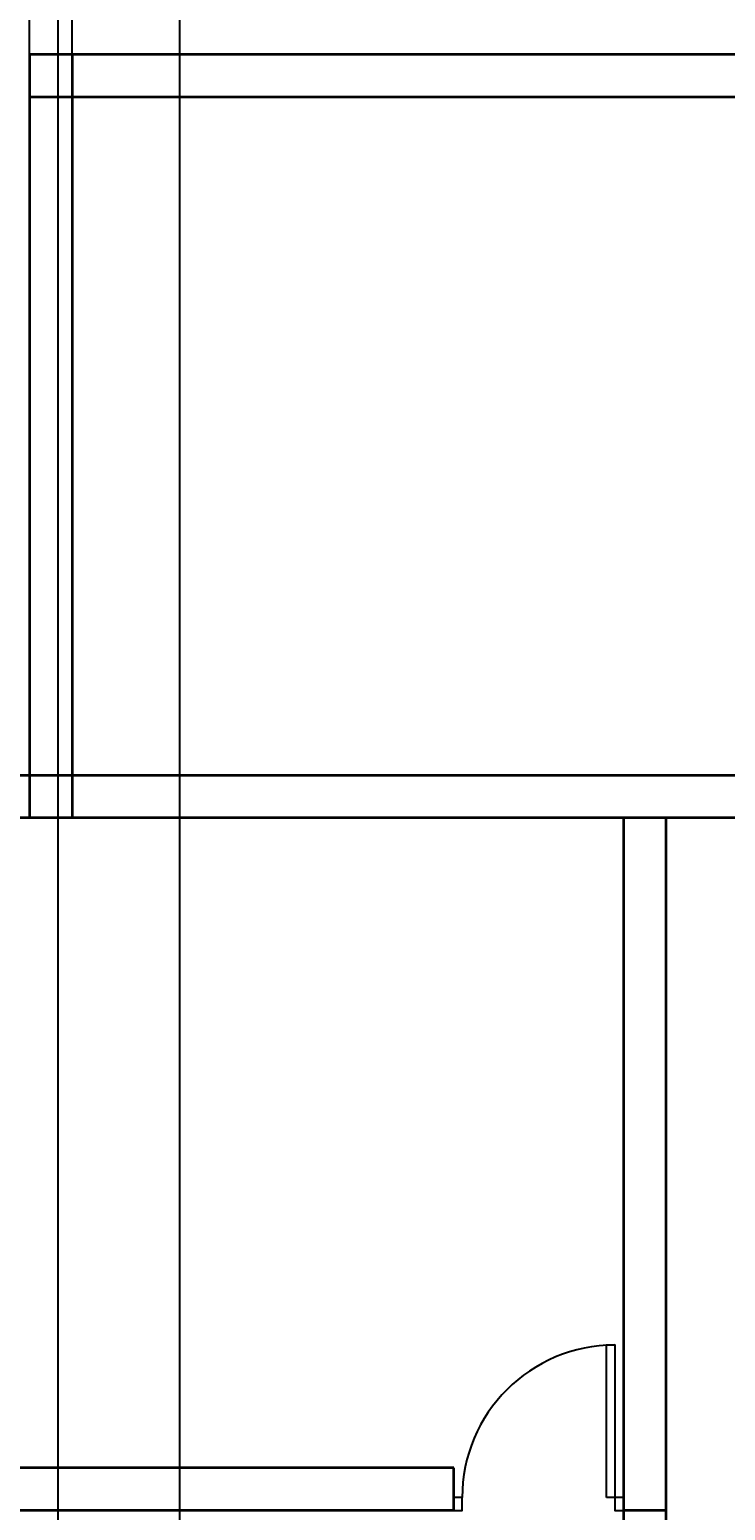
# Model space of a CAD drawing. Units: inches. Extents: x 867 to 1667, y -234 to 788.
# Tile 28 of 42: x 1071 to 1219, y 258 to 572. Entities that reach past the tile are written whole.
import ezdxf

# ---------------------------------------------------------------- set-up
doc = ezdxf.new("R2010")
doc.units = ezdxf.units.IN
doc.header["$MEASUREMENT"] = 0
for name, color, linetype, lineweight in [('A-ANNO-DIMS', 2, 'Continuous', 18), ('A-Door', 150, 'Continuous', 25), ('A-Wall', 7, 'Continuous', 35)]:
    doc.layers.add(name, color=color, linetype=linetype, lineweight=lineweight)
doc.layers.add('NET 01', color=8, linetype='Continuous')
doc.styles.get("Standard").update_dxf_attribs({"font": 'arial.ttf'})
doc.dimstyles.get("Standard").update_dxf_attribs({"dimtxt": 0.6875, "dimasz": 0.18, "dimexe": 0.18, "dimexo": 0.0625, "dimgap": 0.09, "dimtad": 0, "dimdec": 4, "dimzin": 0, "dimdsep": 46, "dimlunit": 4, "dimtxsty": 'Standard', "dimcen": 0.09, "dimadec": 0, "dimazin": 0, "dimtfac": 1, "dimtdec": 4, "dimtofl": 0, "dimtmove": 0, "dimatfit": 3, "dimfxl": 1, "dimtolj": 1, "dimtzin": 0, "dimarcsym": 0})

# ---------------------------------------------------------------- blocks, each defined once
blk = doc.blocks.new('A$C292B336C')
at = {"layer": 'A-Door'}
for points in [[(-0.05, 0), (-0.05, 0.9), (0, 0.9), (0, 0)], [(-0.95, 0), (-0.95, -0.075), (-0.9, -0.075), (-0.9, 0)], [(0, 0), (0, -0.075), (0.05, -0.075), (0.05, 0)]]:
    blk.add_lwpolyline(points, close=True, dxfattribs=at)
at = {"layer": 'NET 01'}
blk.add_arc((0, 0), 0.9, 90, 180, dxfattribs=at)
blk = doc.blocks.new('*D29')
at = {"layer": 'A-ANNO-DIMS', "color": 0, "lineweight": -2, "transparency": 16777216}
for p, q in [((1076.89, 623.55), (1076.89, -233.54)), ((1102.67, 623.55), (1102.67, -233.54)), ((1077.07, -233.36), (1088.52, -233.36)), ((1102.49, -233.36), (1091.03, -233.36))]:
    blk.add_line(p, q, dxfattribs=at)
at = {"layer": 'A-ANNO-DIMS', "color": 0, "transparency": 16777216}
for points in [[(1077.07, -233.33), (1077.07, -233.39), (1076.89, -233.36)], [(1102.49, -233.33), (1102.49, -233.39), (1102.67, -233.36)]]:
    blk.add_solid(points, dxfattribs=at)
at = {"layer": 'Defpoints', "color": 0, "transparency": 16777216}
for p in [(1076.89, 623.62), (1102.67, 623.62), (1102.67, -233.36)]:
    blk.add_point(p, dxfattribs=at)
at = {"layer": 'A-ANNO-DIMS', "color": 0, "transparency": 16777216, "insert": (1089.78, -233.36), "char_height": 0.688, "attachment_point": 5}
blk.add_mtext('\\A1;25.78', dxfattribs=at)
blk = doc.blocks.new('*D31')
at = {"layer": 'A-ANNO-DIMS', "color": 0, "lineweight": -2, "transparency": 16777216}
for p, q in [((1070.89, 566.68), (1070.89, 787.75)), ((1071.07, 787.57), (1304.02, 787.57)), ((1538.71, 787.57), (1305.75, 787.57)), ((1538.89, 566.68), (1538.89, 787.75))]:
    blk.add_line(p, q, dxfattribs=at)
at = {"layer": 'A-ANNO-DIMS', "color": 0, "transparency": 16777216}
for points in [[(1071.07, 787.6), (1071.07, 787.54), (1070.89, 787.57)], [(1538.71, 787.6), (1538.71, 787.54), (1538.89, 787.57)]]:
    blk.add_solid(points, dxfattribs=at)
at = {"layer": 'Defpoints', "color": 0, "transparency": 16777216}
for p in [(1538.89, 787.57), (1070.89, 566.62), (1538.89, 566.62)]:
    blk.add_point(p, dxfattribs=at)
at = {"layer": 'A-ANNO-DIMS', "color": 0, "transparency": 16777216, "insert": (1304.89, 787.57), "char_height": 0.688, "attachment_point": 5}
blk.add_mtext('\\A1;468', dxfattribs=at)
blk = doc.blocks.new('*D32')
at = {"layer": 'A-ANNO-DIMS', "color": 0, "lineweight": -2, "transparency": 16777216}
for p, q in [((1079.89, 404.68), (1079.89, 787.75)), ((1080.07, 787.57), (1163.07, 787.57)), ((1247.71, 787.57), (1164.7, 787.57)), ((1247.89, 413.68), (1247.89, 787.75))]:
    blk.add_line(p, q, dxfattribs=at)
at = {"layer": 'A-ANNO-DIMS', "color": 0, "transparency": 16777216}
for points in [[(1080.07, 787.6), (1080.07, 787.54), (1079.89, 787.57)], [(1247.71, 787.6), (1247.71, 787.54), (1247.89, 787.57)]]:
    blk.add_solid(points, dxfattribs=at)
at = {"layer": 'Defpoints', "color": 0, "transparency": 16777216}
for p in [(1247.89, 787.57), (1247.89, 413.62), (1079.89, 404.62)]:
    blk.add_point(p, dxfattribs=at)
at = {"layer": 'A-ANNO-DIMS', "color": 0, "transparency": 16777216, "insert": (1163.89, 787.57), "char_height": 0.688, "attachment_point": 5}
blk.add_mtext('\\A1;168', dxfattribs=at)

msp = doc.modelspace()

# ---------------------------------------------------------------- linework, layer by layer
at = {"layer": 'A-Wall'}
for p, q in [((1538.8866, 566.617), (1070.8866, 566.617)), ((1070.8866, 566.617), (1070.8866, 404.617)), ((1079.8866, 566.617), (1079.8866, 404.617)), ((1538.8866, 557.617), (1070.8866, 557.617)), ((1529.8866, 413.617), (1040.8866, 413.617)), ((1559.8866, 404.617), (1040.8866, 404.617)), ((1196.8866, 404.617), (1196.8866, 136.117)), ((1205.8866, 404.617), (1205.8866, 136.117)), ((1160.8866, 266.617), (1040.8866, 266.617)), ((1160.8866, 257.617), (1160.8866, 266.617)), ((1160.8866, 257.617), (1040.8866, 257.617)), ((1205.8866, 257.617), (1196.8866, 257.617))]:
    msp.add_line(p, q, dxfattribs=at)

# ---------------------------------------------------------------- block references
at = {"layer": 'A-Door', "xscale": 36.01171521992244, "yscale": 36.01171521992244, "zscale": 36.01171521992244}
msp.add_blockref('A$C292B336C', (1195.086, 260.3179), dxfattribs=at)

# ---------------------------------------------------------------- dimensions: what is measured, and where the dimension line sits
at = {"layer": 'A-ANNO-DIMS'}
for base, p1, p2, override, picture, middle in [((1538.8866, 787.567), (1070.8866, 566.617), (1538.8866, 566.617), {"dimdec": 0, "dimlfac": 1, "dimrnd": 0, "dimzin": 0, "dimdsep": 46, "dimlunit": 2}, '*D31', (1304.8866, 787.567)), ((1247.8866, 787.567), (1079.8866, 404.617), (1247.8866, 413.617), {"dimdec": 0, "dimlfac": 1, "dimrnd": 0, "dimzin": 0, "dimdsep": 46, "dimlunit": 2}, '*D32', (1163.8866, 787.567)), ((1102.6661, -233.3581), (1076.8866, 623.617), (1102.6661, 623.617), {"dimdec": 2, "dimlfac": 1, "dimrnd": 0, "dimzin": 0, "dimdsep": 46, "dimlunit": 2}, '*D29', (1089.7763, -233.3581))]:
    dim = msp.add_linear_dim(base=base, p1=p1, p2=p2, dimstyle='Standard', override=override, dxfattribs=at)
    dim.commit()
    dim.dimension.update_dxf_attribs({"geometry": picture, "text_midpoint": middle})

doc.saveas('drawing.dxf')
